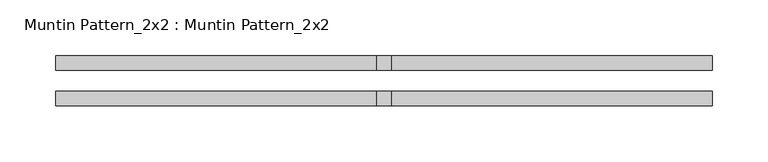
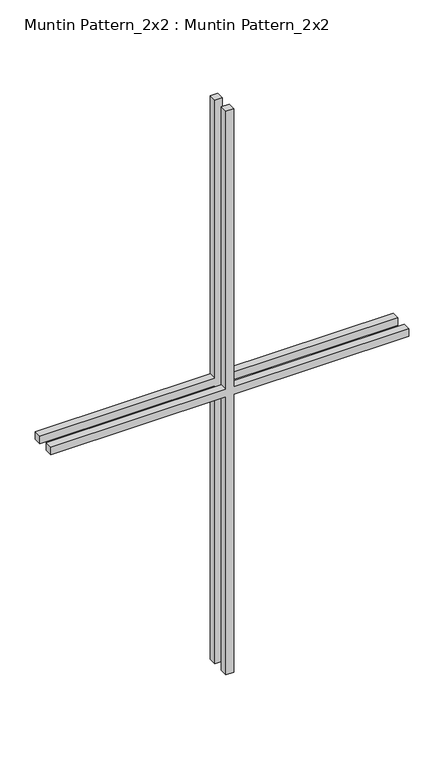
"""IFC4 building model written with IfcOpenShell, lengths in millimetres: proxy geometry, Muntin Pattern_2x2 : Muntin Pattern_2x2."""

from ifc_helpers import new_model, si_unit, frame, origin, place, context, project, spatial, polyline, outline, extrude, source, transform, mapped, element, save


def muntin_pattern_2x2_muntin_pattern_2x2_11ff06db(model_context):
    return source(origin(), model_context, "Body", "SweptSolid", [
        extrude(outline(polyline([(495.3, -6.35), (495.3, -293.6875), (482.6, -293.6875), (482.6, -6.35), (0.0, -6.35), (0.0, 6.35), (482.6, 6.35), (482.6, 293.6875), (495.3, 293.6875), (495.3, 6.35), (977.9, 6.35), (977.9, -6.35), (495.3, -6.35)])), frame((0.0, -22.225, 0.0), z_axis=(0.0, 1.0, 0.0), x_axis=(0.0, 0.0, 1.0)), (0.0, 0.0, 1.0), 12.7),
        extrude(outline(polyline([(495.3, -6.35), (495.3, -293.6875), (482.6, -293.6875), (482.6, -6.35), (0.0, -6.35), (0.0, 6.35), (482.6, 6.35), (482.6, 293.6875), (495.3, 293.6875), (495.3, 6.35), (977.9, 6.35), (977.9, -6.35), (495.3, -6.35)])), frame((0.0, 9.525, 0.0), z_axis=(0.0, 1.0, 0.0), x_axis=(0.0, 0.0, 1.0)), (0.0, 0.0, 1.0), 12.7),
    ])


if __name__ == "__main__":
    model = new_model("IFC4")
    model_context = context("Model", 3, world=origin())
    ifc_project = project(units=[si_unit("LENGTHUNIT", "METRE", prefix="MILLI")], contexts=[model_context])
    site = spatial("IfcSite", under=ifc_project)
    building = spatial("IfcBuilding", under=site)
    placement = place(None, origin())
    muntin_pattern_2x2_muntin_pattern_2x2_shape = muntin_pattern_2x2_muntin_pattern_2x2_11ff06db(model_context)
    element("IfcBuildingElementProxy", 1, Name="Muntin Pattern_2x2 : Muntin Pattern_2x2", ObjectType="Muntin Pattern_2x2 : Muntin Pattern_2x2", at=placement, inside=building, context=model_context, shape_type="MappedRepresentation", body=[
        mapped(muntin_pattern_2x2_muntin_pattern_2x2_shape, transform((0.0, 0.0, 0.0), x_axis=(1.0, 0.0, 0.0), y_axis=(0.0, 1.0, 0.0), z_axis=(0.0, 0.0, 1.0))),
    ])
    save(model, "model.ifc")

# Revit data of these elements
# Type "Muntin Pattern_2x2 : Muntin Pattern_2x2"
#   Width [instance default] = 48"
#   Thickness = 0.5"
#   Height [instance default] = 48"
#   Distance = 0.75"
#   Interior Material [instance default] = none
#   Exterior Material [instance default] = none
#   Default Elevation = 0
# Element 1 (IfcBuildingElementProxy, "Muntin Pattern_2x2 : Muntin Pattern_2x2")
#   Width = 23.125"
#   Height = 38.5"
#   Interior Material = Wood - Stained
#   Exterior Material = Clad - White
#   Materials on its faces: "Clad - White", "Wood - Stained"
# Materials
#   "Clad - White": class "Wood", colour RGB 242 242 238, transparency 0, Cost = 0
#   "Wood - Stained": class "Wood", colour RGB 224 178 126, transparency 0, Cost = 0
